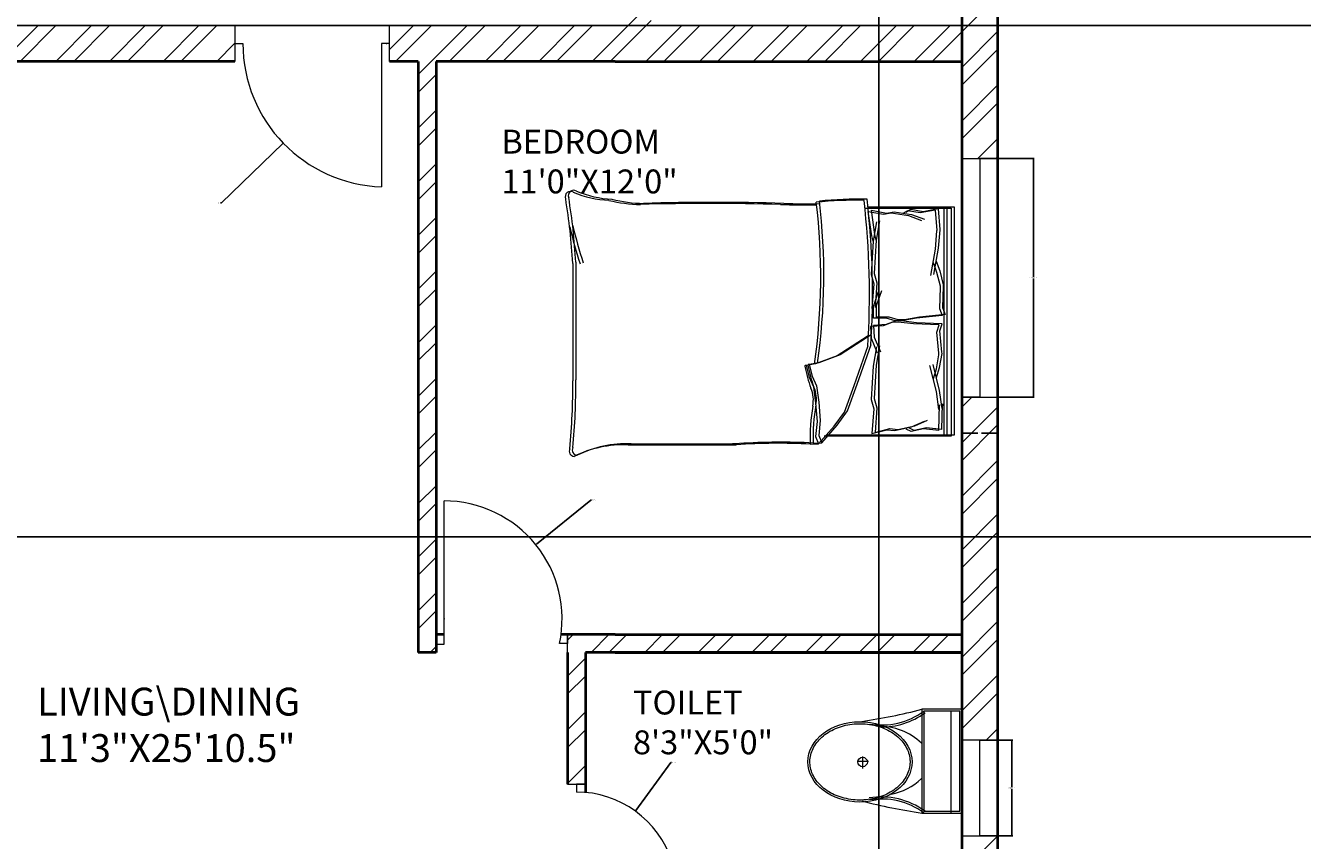
# Model space of a CAD drawing. Units: inches. Extents: x 1355 to 2746, y 1171 to 2751.
# Tile 4 of 24: x 1697 to 2017, y 1482 to 1686. Entities that reach past the tile are written whole.
import ezdxf

# ---------------------------------------------------------------- set-up
doc = ezdxf.new("R2010")
doc.units = ezdxf.units.IN
for name, color, linetype, lineweight in [('A-ANNO-DIMS', 2, 'Continuous', 18), ('A-AREA-IDEN', 7, 'Continuous', 18), ('A-DOOR', 3, 'Continuous', 20), ('A-FLOR-FIXT', 9, 'Continuous', 18), ('A-FURN', 8, 'Continuous', 13), ('A-GLAZ', 4, 'Continuous', 18), ('A-WALL', 7, 'Continuous', 40), ('A-WALL-PATT', 252, 'Continuous', 13)]:
    doc.layers.add(name, color=color, linetype=linetype, lineweight=lineweight)
doc.styles.get("Standard").update_dxf_attribs({"font": 'arial.ttf'})
doc.dimstyles.get("Standard").update_dxf_attribs({"dimtxt": 0.18, "dimasz": 0.18, "dimexe": 0.18, "dimexo": 0.0625, "dimgap": 0.09, "dimtad": 0, "dimtih": 1, "dimtoh": 1, "dimdec": 4, "dimzin": 0, "dimdsep": 46, "dimtxsty": 'Standard', "dimcen": 0.09, "dimadec": 0, "dimazin": 0, "dimtfac": 1, "dimtdec": 4, "dimtofl": 0, "dimtmove": 0, "dimatfit": 3, "dimfxl": 1, "dimtolj": 1, "dimtzin": 0, "dimarcsym": 0})

# ---------------------------------------------------------------- blocks, each defined once
blk = doc.blocks.new('A$C31115884')
for p, q in [((257.5, 466.4), (257.5, 523.2)), ((283.1, 497.7), (223.4, 497.7)), ((0, 200), (0, 0)), ((520, 200), (0, 200)), ((520, 0), (520, 200)), ((10, 190), (10, 10)), ((510, 190), (10, 190)), ((510, 10), (510, 190)), ((510, 54.5), (0, 54.5)), ((10, 10), (510, 10)), ((0, 0), (520, 0))]:
    blk.add_line(p, q)
blk.add_circle((255.6, 496.4), 23.6)
for centre, radius, start, end in [((2777.7, -204.6), 2807, 165.4549, 171.71327), ((-294.5, 403.3), 364.7, 324.20913, 9.34987), ((-294.5, 403.3), 374.7, 324.20913, 9.34987), ((805.8, 403.3), 364.7, 170.65013, 215.79087), ((3237, 905), 2807, 188.28673, 194.5451), ((139.5, 406.2), 293.5, 315.84364, 2.65635), ((805.8, 403.3), 374.7, 179.20365, 215.79087), ((383.6, 406.2), 293.5, 190.27735, 224.15636)]:
    blk.add_arc(centre, radius, start, end)
blk.add_ellipse((256.2, 509.9), major_axis=(0, -260.7), ratio=0.772727)
blk.add_open_spline([(256.2, 259.2), (263.1, 259.2), (270, 259.7), (287.8, 262.3), (298.7, 265.1), (319.9, 273.1), (330.2, 278.4), (350.1, 291.1), (359.7, 298.7), (377.7, 315.9), (386.2, 325.5), (401.7, 346.6), (408.8, 358.1), (421.3, 382.5), (426.8, 395.5), (435.9, 422.4), (439.5, 436.4), (444.8, 465.1), (446.5, 479.7), (447.9, 509.2), (447.6, 524), (445, 553.3), (442.7, 567.8), (436.3, 596), (432.1, 609.7), (421.9, 636), (416, 648.6), (402.5, 672.1), (395, 683), (378.6, 703), (369.8, 712.1), (351.1, 728), (341.3, 734.8), (320.9, 746.2), (310.4, 750.7), (288.9, 757.3), (278, 759.4), (256, 761), (245, 760.6), (223.1, 757.2), (212.3, 754.3), (191.1, 746.1), (180.8, 740.7), (160.9, 727.8), (151.4, 720.1), (133.5, 702.7), (125.1, 693), (109.6, 671.7), (102.6, 660.2), (90.2, 635.7), (84.9, 622.7), (76, 595.6), (72.4, 581.6), (67.2, 552.9), (65.6, 538.2), (64.4, 508.8), (64.8, 494), (67.5, 464.7), (69.9, 450.2), (76.6, 422), (80.8, 408.3), (91.1, 382.2), (97.2, 369.7), (110.8, 346.3), (118.4, 335.4), (134.8, 315.6), (143.7, 306.7), (162.4, 290.9), (172.3, 284.2), (192.8, 273), (203.3, 268.6), (224.8, 262.2), (235.8, 260.2), (249.9, 259.3), (253, 259.2), (256.2, 259.2)], degree=3, knots=[0, 0, 0, 0, 0.110105, 0.110105, 0.285049, 0.285049, 0.459994, 0.459994, 0.634938, 0.634938, 0.809882, 0.809882, 0.984827, 0.984827, 1.159771, 1.159771, 1.334715, 1.334715, 1.50966, 1.50966, 1.684604, 1.684604, 1.859549, 1.859549, 2.034493, 2.034493, 2.209437, 2.209437, 2.384382, 2.384382, 2.559326, 2.559326, 2.73427, 2.73427, 2.909215, 2.909215, 3.084159, 3.084159, 3.259103, 3.259103, 3.434048, 3.434048, 3.608992, 3.608992, 3.783936, 3.783936, 3.958881, 3.958881, 4.133825, 4.133825, 4.30877, 4.30877, 4.483714, 4.483714, 4.658658, 4.658658, 4.833603, 4.833603, 5.008547, 5.008547, 5.183491, 5.183491, 5.358436, 5.358436, 5.53338, 5.53338, 5.708324, 5.708324, 5.883269, 5.883269, 6.058213, 6.058213, 6.233158, 6.233158, 6.283185, 6.283185, 6.283185, 6.283185])
blk = doc.blocks.new('BED-DOUBLE-PLAN')
for p, q in [((75.16, 62.38), (96.87, 62.38)), ((75.93, 62.66), (97.64, 62.66)), ((76.95, 55.42), (76.08, 61.53)), ((76.08, 61.53), (79.9, 60.84)), ((77.72, 55.7), (76.85, 61.81)), ((76.85, 61.81), (80.66, 61.11)), ((79.9, 60.84), (81.8, 61.19)), ((80.66, 61.11), (82.57, 61.46)), ((81.8, 61.19), (86.14, 60.49)), ((82.57, 61.46), (86.9, 60.77)), ((85.96, 61.71), (84.75, 61.01)), ((86.73, 61.98), (85.52, 61.29)), ((89.08, 61.19), (85.96, 61.71)), ((89.85, 61.46), (86.73, 61.98)), ((92.9, 61.88), (89.08, 61.19)), ((93.66, 62.15), (89.85, 61.46)), ((92.87, 61.87), (93.27, 56.74)), ((93.64, 62.15), (94.03, 57.02)), ((95.03, 62.38), (95.03, 5.09)), ((95.8, 62.66), (95.8, 5.36)), ((96.87, 62.38), (96.87, 5.09)), ((97.64, 62.66), (97.64, 5.36)), ((78.14, 58.9), (77.34, 54.06)), ((78.9, 59.17), (78.1, 54.34)), ((86.14, 60.49), (89.43, 59.28)), ((86.9, 60.77), (90.2, 59.55)), ((77.34, 54.06), (76.95, 55.42)), ((78.1, 54.34), (77.72, 55.7)), ((93.24, 56.62), (92.9, 52.03)), ((93.27, 56.74), (93.24, 56.62)), ((94.01, 56.89), (93.66, 52.31)), ((94.03, 57.02), (94.01, 56.89)), ((77.34, 54.06), (76.82, 45.66)), ((78.1, 54.34), (77.59, 45.93)), ((92.9, 52.03), (91.68, 45.45)), ((93.66, 52.31), (92.45, 45.72)), ((1.87, 48.49), (1.87, 18.98)), ((2.64, 48.76), (2.64, 19.26)), ((92.38, 48.74), (93.24, 46.31)), ((93.14, 49.01), (94.01, 46.59)), ((76.82, 45.66), (77.49, 43.31)), ((77.59, 45.93), (78.25, 43.58)), ((93.24, 46.31), (94.11, 42.85)), ((94.01, 46.59), (94.88, 43.12)), ((77.49, 43.31), (77, 37.16)), ((78.25, 43.58), (77.77, 37.43)), ((78.14, 37.93), (79.45, 41.7)), ((94.11, 42.46), (93.94, 37.13)), ((94.11, 42.85), (94.11, 42.46)), ((94.88, 42.74), (94.7, 37.41)), ((94.88, 43.12), (94.88, 42.74)), ((77.38, 37.65), (78.68, 41.42)), ((77.38, 34.71), (77.38, 37.65)), ((78.14, 34.98), (78.14, 37.93)), ((94.63, 35.4), (88.22, 34.71)), ((95.4, 35.67), (88.98, 34.98)), ((93.94, 37.13), (94.63, 35.4)), ((94.7, 37.41), (95.4, 35.67)), ((79.83, 32.82), (76.62, 32.62)), ((76.62, 32.62), (76.8, 29.68)), ((80.59, 34.71), (77.38, 34.71)), ((80.6, 33.1), (77.39, 32.9)), ((77.39, 32.9), (77.57, 29.96)), ((81.36, 34.98), (78.14, 34.98)), ((82.03, 33.66), (79.83, 32.82)), ((82.84, 34.01), (80.59, 34.71)), ((82.8, 33.93), (80.6, 33.1)), ((83.61, 34.29), (81.36, 34.98)), ((83.59, 33.75), (82.03, 33.66)), ((84.36, 34.03), (82.8, 33.93)), ((84.4, 34.01), (82.84, 34.01)), ((87.44, 33.3), (83.59, 33.75)), ((85.17, 34.29), (83.61, 34.29)), ((88.21, 33.57), (84.36, 34.03)), ((88.22, 34.71), (84.4, 34.01)), ((88.98, 34.98), (85.17, 34.29)), ((93.89, 33.01), (87.44, 33.3)), ((94.65, 33.28), (88.21, 33.57)), ((93.3, 31.24), (93.89, 33.01)), ((94.07, 31.51), (94.65, 33.28)), ((76.03, 30.27), (68.25, 25.25)), ((76.8, 30.55), (69.01, 25.52)), ((76.8, 29.68), (78.34, 26)), ((77.57, 29.96), (79.11, 26.28)), ((93.81, 25.93), (93.3, 31.24)), ((94.57, 26.2), (94.07, 31.51)), ((72.52, 17.82), (76.03, 27.82)), ((73.28, 18.1), (76.8, 28.09)), ((78.14, 27.51), (77.34, 22.68)), ((78.9, 27.78), (78.1, 22.95)), ((93.83, 25.54), (93.81, 25.93)), ((93.95, 22.3), (94.6, 25.82)), ((94.6, 25.82), (94.57, 26.2)), ((62.87, 23.21), (60.45, 22.84)), ((60.45, 22.84), (61.2, 19.86)), ((63.63, 23.48), (61.22, 23.11)), ((61.22, 23.11), (61.96, 20.14)), ((68.25, 25.25), (62.87, 23.21)), ((69.01, 25.52), (63.63, 23.48)), ((77.34, 22.68), (76.82, 14.27)), ((78.1, 22.95), (77.59, 14.54)), ((93.19, 16.3), (91.57, 22.8)), ((93.96, 16.57), (92.34, 23.07)), ((93.18, 22.03), (93.83, 25.54)), ((61.2, 19.86), (62.31, 17.45)), ((61.96, 20.14), (63.08, 17.72)), ((92.47, 19.55), (93.18, 22.03)), ((93.23, 19.83), (93.95, 22.3)), ((62.31, 17.45), (62.87, 13.37)), ((63.08, 17.72), (63.63, 13.64)), ((70.1, 11.14), (72.52, 17.82)), ((70.87, 11.41), (73.28, 18.1)), ((93.82, 11.75), (93.19, 16.3)), ((94.59, 12.02), (93.96, 16.57)), ((62.87, 13.37), (63.24, 8.72)), ((63.63, 13.64), (64, 9)), ((76.82, 14.27), (77.49, 11.92)), ((77.59, 14.54), (78.25, 12.19)), ((93.81, 6.47), (93.92, 12.95)), ((93.92, 12.95), (93.82, 11.75)), ((94.57, 6.75), (94.69, 13.22)), ((94.69, 13.22), (94.59, 12.02)), ((67.51, 7.61), (70.1, 11.14)), ((68.27, 7.88), (70.87, 11.41)), ((77.49, 11.92), (77, 5.77)), ((78.25, 12.19), (77.77, 6.04)), ((63.24, 8.72), (62.87, 5.01)), ((63.61, 3.17), (67.51, 7.61)), ((64, 9), (63.63, 5.28)), ((64.38, 3.44), (68.27, 7.88)), ((77, 5.77), (80.77, 6.7)), ((77.77, 6.04), (81.53, 6.97)), ((80.77, 6.7), (82.69, 6.47)), ((81.53, 6.97), (83.46, 6.75)), ((82.69, 6.47), (86.97, 7.43)), ((83.46, 6.75), (87.74, 7.71)), ((86.88, 6.21), (85.62, 6.83)), ((87.64, 6.49), (86.39, 7.1)), ((89.96, 6.93), (86.88, 6.21)), ((86.97, 7.43), (90.18, 8.85)), ((90.72, 7.2), (87.64, 6.49)), ((87.74, 7.71), (90.95, 9.12)), ((93.81, 6.47), (89.96, 6.93)), ((94.57, 6.75), (90.72, 7.2)), ((62.28, 3.35), (64.38, 3.44, 4.64)), ((62.87, 5.01), (63.61, 3.17)), ((63.63, 5.28), (64.38, 3.44)), ((96.87, 5.09), (64.97, 5.09)), ((97.64, 5.36), (65.74, 5.36)), ((61.52, 3.07), (63.61, 3.17, 4.64))]:
    blk.add_line(p, q)
for centre, radius, start, end in [((1.3, 65.24), 1.31, 56.1736, 203.4781), ((-143.9, 40.86), 145.97, 2.9958, 9.4091), ((2.07, 65.52), 1.31, 56.1736, 203.4781), ((-143.14, 41.13), 145.97, 2.9958, 9.4091), ((12.62, 92.52), 28.25, 247.9751, 266.652), ((13.39, 92.79), 28.25, 247.9751, 266.652), ((19.53, 98.8), 35.53, 256.0648, 268.9113), ((20.29, 99.07), 35.53, 256.0648, 268.9113), ((72.78, -35.55), 99.87, 88.7218, 95.604), ((73.55, -35.27), 99.87, 88.7218, 95.604), ((-121.38, 40.94), 197.77, 356.0865, 6.7821), ((-120.62, 41.22), 197.77, 356.0865, 6.7821), ((36.19, -514.68), 578.22, 88.22771, 91.71854), ((36.96, -514.41), 578.22, 88.22771, 91.71854), ((59.5, 267.13), 203.94, 268.4762, 271.0082), ((60.27, 267.4), 203.94, 268.4762, 271.0082), ((-90.53, 45.26), 154.68, 351.7845, 6.9006), ((-89.76, 45.54), 154.68, 351.7845, 6.9006), ((126.07, 87.47), 127.63, 193.3832, 197.7053), ((125.3, 87.2), 127.63, 193.3832, 197.7053), ((60.38, 22.63), 0.221, 70.2464, 181.1377), ((95.1, 29.2), 35.55, 190.6617, 199.8806), ((61.15, 22.9), 0.221, 70.2464, 181.1377), ((95.86, 29.47), 35.55, 190.6617, 199.8806), ((-156.85, 17.49), 159.5, 354.4998, 0.6351), ((-157.62, 17.21), 159.5, 354.4998, 0.6351), ((54.83, 14.11), 7.46, 348.6608, 23.7384), ((55.6, 14.38), 7.46, 348.6608, 23.7384), ((105.62, 5.29), 43.38, 169.8763, 182.5657), ((104.85, 5.01), 43.38, 169.8763, 182.5657), ((16.33, 5472.16), 5469.02, 270.00217, 270.28689), ((53.34, -151.96), 155.25, 86.9791, 93.8365), ((54.1, -151.69), 155.25, 86.9791, 93.8365), ((2.32, 1.32), 1.32, 152.6588, 266.02), ((3.08, 1.59), 1.32, 152.6588, 266.02), ((14.55, -24.75), 27.65, 87.4714, 116.4681), ((15.32, -24.48), 27.65, 87.4714, 116.4681), ((15.56, 5471.89), 5469.02, 270.00217, 270.28689)]:
    blk.add_arc(centre, radius, start, end)
blk = doc.blocks.new('WINDOW-PLAN-60')
for p, q in [((0, 60), (9, 60)), ((9, 60), (4.5, 60)), ((4.5, 60), (4.5, 0)), ((4.5, 0), (0, 0)), ((0, 0), (9, 0))]:
    blk.add_line(p, q)
blk = doc.blocks.new('WINDOW-PLAN-24-3')
for p, q in [((9, 24), (0, 24)), ((0, 24), (0, 24)), ((4.5, 0), (4.5, 24)), ((4.5, 24), (9, 24)), ((0, 0), (9, 0)), ((9, 0), (4.5, 0))]:
    blk.add_line(p, q)
blk = doc.blocks.new('DOOR-BED-SE')
for p, q in [((2, 2.1), (2, 38.1)), ((33, 0), (33, 4.5)), ((33, 4.5), (33, 2.25)), ((0, 2.1), (2, 2.1)), ((33, 2.25), (31, 2.25))]:
    blk.add_line(p, q)
blk.add_arc((2, 8.44), 29.65, 347.948, 90)
blk = doc.blocks.new('DOOR-WC-SE')
for p, q in [((0, 21.41), (4.5, 21.41)), ((4.5, 21.41), (2.25, 21.41)), ((2.25, 21.41), (2.25, 19.41)), ((2.25, 0), (2.25, 2)), ((2.25, 2), (26.25, 2)), ((4.5, 0), (0, 0)), ((0, 0), (2.25, 0))]:
    blk.add_line(p, q)
blk.add_arc((2.25, -5.83), 25.25, 18.0786, 90)
blk = doc.blocks.new('DOOR-ENTRY-S')
for p, q in [((0, 40.5), (0, 31.5)), ((38.81, 31.5), (38.81, 40.5)), ((0, 36), (2, 36)), ((38.81, 36), (36.81, 36)), ((36.81, 36), (36.81, 0))]:
    blk.add_line(p, q)
blk.add_arc((38.02, 36), 36.02, 180, 268.0706)
blk = doc.blocks.new('*D39')
at = {"layer": 'A-ANNO-DIMS', "color": 0, "lineweight": -2, "transparency": 16777216}
for p, q in [((1940.77, 1652.94), (1949.89, 1652.94)), ((1949.71, 1652.76), (1949.71, 1623.13)), ((1949.71, 1593.12), (1949.71, 1622.76)), ((1940.77, 1592.94), (1949.89, 1592.94))]:
    blk.add_line(p, q, dxfattribs=at)
at = {"layer": 'A-ANNO-DIMS', "color": 0, "transparency": 16777216}
for points in [[(1949.68, 1652.76), (1949.74, 1652.76), (1949.71, 1652.94)], [(1949.68, 1593.12), (1949.74, 1593.12), (1949.71, 1592.94)]]:
    blk.add_solid(points, dxfattribs=at)
at = {"layer": 'Defpoints', "color": 0, "transparency": 16777216}
for p in [(1940.71, 1652.94), (1949.71, 1652.94), (1940.71, 1592.94)]:
    blk.add_point(p, dxfattribs=at)
at = {"layer": 'A-ANNO-DIMS', "color": 0, "transparency": 16777216, "insert": (1949.71, 1622.94), "char_height": 0.18, "attachment_point": 5}
blk.add_mtext('\\A1;WINDOW 60 TYP.', dxfattribs=at)
blk = doc.blocks.new('*D40')
at = {"layer": 'A-ANNO-DIMS', "color": 0, "lineweight": -2, "transparency": 16777216}
for p, q in [((1931.71, 1592.88), (1931.71, 1583.76)), ((1940.71, 1592.88), (1940.71, 1583.76)), ((1931.89, 1583.94), (1935.75, 1583.94)), ((1940.53, 1583.94), (1936.67, 1583.94))]:
    blk.add_line(p, q, dxfattribs=at)
at = {"layer": 'A-ANNO-DIMS', "color": 0, "transparency": 16777216}
for points in [[(1931.89, 1583.97), (1931.89, 1583.91), (1931.71, 1583.94)], [(1940.53, 1583.97), (1940.53, 1583.91), (1940.71, 1583.94)]]:
    blk.add_solid(points, dxfattribs=at)
at = {"layer": 'Defpoints', "color": 0, "transparency": 16777216}
for p in [(1931.71, 1592.94), (1940.71, 1592.94), (1940.71, 1583.94)]:
    blk.add_point(p, dxfattribs=at)
at = {"layer": 'A-ANNO-DIMS', "color": 0, "transparency": 16777216, "insert": (1936.21, 1583.94), "char_height": 0.18, "attachment_point": 5}
blk.add_mtext('\\A1;9 TYP.', dxfattribs=at)
blk = doc.blocks.new('*D51')
at = {"layer": 'A-ANNO-DIMS', "color": 0, "lineweight": -2, "transparency": 16777216}
for p, q in [((1940.77, 1506.78), (1944.49, 1506.78)), ((1944.31, 1506.6), (1944.31, 1494.97)), ((1944.31, 1482.96), (1944.31, 1494.6)), ((1940.77, 1482.78), (1944.49, 1482.78))]:
    blk.add_line(p, q, dxfattribs=at)
at = {"layer": 'A-ANNO-DIMS', "color": 0, "transparency": 16777216}
for points in [[(1944.28, 1506.6), (1944.34, 1506.6), (1944.31, 1506.78)], [(1944.28, 1482.96), (1944.34, 1482.96), (1944.31, 1482.78)]]:
    blk.add_solid(points, dxfattribs=at)
at = {"layer": 'Defpoints', "color": 0, "transparency": 16777216}
for p in [(1940.71, 1506.78), (1944.31, 1506.78), (1940.71, 1482.78)]:
    blk.add_point(p, dxfattribs=at)
at = {"layer": 'A-ANNO-DIMS', "color": 0, "transparency": 16777216, "insert": (1944.31, 1494.78), "char_height": 0.18, "attachment_point": 5}
blk.add_mtext('\\A1;WINDOW 24 TYP.', dxfattribs=at)
blk = doc.blocks.new('*D52')
at = {"layer": 'A-ANNO-DIMS', "color": 0, "lineweight": -2, "transparency": 16777216}
for p, q in [((1931.71, 1482.72), (1931.71, 1479)), ((1940.71, 1482.72), (1940.71, 1479)), ((1931.89, 1479.18), (1935.75, 1479.18)), ((1940.53, 1479.18), (1936.67, 1479.18))]:
    blk.add_line(p, q, dxfattribs=at)
at = {"layer": 'A-ANNO-DIMS', "color": 0, "transparency": 16777216}
for points in [[(1931.89, 1479.21), (1931.89, 1479.15), (1931.71, 1479.18)], [(1940.53, 1479.21), (1940.53, 1479.15), (1940.71, 1479.18)]]:
    blk.add_solid(points, dxfattribs=at)
at = {"layer": 'Defpoints', "color": 0, "transparency": 16777216}
for p in [(1931.71, 1482.78), (1940.71, 1482.78), (1940.71, 1479.18)]:
    blk.add_point(p, dxfattribs=at)
at = {"layer": 'A-ANNO-DIMS', "color": 0, "transparency": 16777216, "insert": (1936.21, 1479.18), "char_height": 0.18, "attachment_point": 5}
blk.add_mtext('\\A1;9 TYP.', dxfattribs=at)
blk = doc.blocks.new('*D106')
at = {"layer": 'A-ANNO-DIMS', "color": 0, "lineweight": -2, "transparency": 16777216}
for p, q in [((2031.09, 1557.85), (1407.53, 1557.85)), ((1407.71, 1557.67), (1407.71, 1434.76)), ((1407.71, 1311.48), (1407.71, 1434.39)), ((2080.33, 1311.3), (1407.53, 1311.3))]:
    blk.add_line(p, q, dxfattribs=at)
at = {"layer": 'A-ANNO-DIMS', "color": 0, "transparency": 16777216}
for points in [[(1407.68, 1557.67), (1407.74, 1557.67), (1407.71, 1557.85)], [(1407.68, 1311.48), (1407.74, 1311.48), (1407.71, 1311.3)]]:
    blk.add_solid(points, dxfattribs=at)
at = {"layer": 'Defpoints', "color": 0, "transparency": 16777216}
for p in [(1407.71, 1557.85), (2031.15, 1557.85), (2080.39, 1311.3)]:
    blk.add_point(p, dxfattribs=at)
at = {"layer": 'A-ANNO-DIMS', "color": 0, "transparency": 16777216, "insert": (1407.71, 1434.57), "char_height": 0.18, "attachment_point": 5}
blk.add_mtext('\\A1;246.54', dxfattribs=at)
blk = doc.blocks.new('*D107')
at = {"layer": 'A-ANNO-DIMS', "color": 0, "lineweight": -2, "transparency": 16777216}
for p, q in [((2089.33, 1686.3), (1407.53, 1686.3)), ((1407.71, 1686.12), (1407.71, 1622.26)), ((1407.71, 1558.03), (1407.71, 1621.89)), ((2031.09, 1557.85), (1407.53, 1557.85))]:
    blk.add_line(p, q, dxfattribs=at)
at = {"layer": 'A-ANNO-DIMS', "color": 0, "transparency": 16777216}
for points in [[(1407.68, 1686.12), (1407.74, 1686.12), (1407.71, 1686.3)], [(1407.68, 1558.03), (1407.74, 1558.03), (1407.71, 1557.85)]]:
    blk.add_solid(points, dxfattribs=at)
at = {"layer": 'Defpoints', "color": 0, "transparency": 16777216}
for p in [(1407.71, 1686.3), (2089.39, 1686.3), (2031.15, 1557.85)]:
    blk.add_point(p, dxfattribs=at)
at = {"layer": 'A-ANNO-DIMS', "color": 0, "transparency": 16777216, "insert": (1407.71, 1622.07), "char_height": 0.18, "attachment_point": 5}
blk.add_mtext('\\A1;128.46', dxfattribs=at)
blk = doc.blocks.new('*D145')
at = {"layer": 'A-ANNO-DIMS', "color": 0, "lineweight": -2, "transparency": 16777216}
for p, q in [((1910.88, 1399.86), (1910.88, 2716.58)), ((1911.06, 2716.4), (1920.83, 2716.4)), ((1931.53, 2716.4), (1921.76, 2716.4)), ((1931.71, 1399.86), (1931.71, 2716.58))]:
    blk.add_line(p, q, dxfattribs=at)
at = {"layer": 'A-ANNO-DIMS', "color": 0, "transparency": 16777216}
for points in [[(1911.06, 2716.43), (1911.06, 2716.37), (1910.88, 2716.4)], [(1931.53, 2716.43), (1931.53, 2716.37), (1931.71, 2716.4)]]:
    blk.add_solid(points, dxfattribs=at)
at = {"layer": 'Defpoints', "color": 0, "transparency": 16777216}
for p in [(1931.71, 2716.4), (1910.88, 1399.8), (1931.71, 1399.8)]:
    blk.add_point(p, dxfattribs=at)
at = {"layer": 'A-ANNO-DIMS', "color": 0, "transparency": 16777216, "insert": (1921.3, 2716.4), "char_height": 0.18, "attachment_point": 5}
blk.add_mtext('\\A1;20.824', dxfattribs=at)
blk = doc.blocks.new('*D155')
at = {"layer": 'A-ANNO-DIMS', "color": 0, "lineweight": -2, "transparency": 16777216}
for p, q in [((1787.15, 1681.8), (1787.33, 1681.8)), ((1787.24, 1681.71), (1787.24, 1681.89)), ((1745.81, 1641.74), (1761.22, 1656.64)), ((1745.63, 1641.74), (1745.81, 1641.74))]:
    blk.add_line(p, q, dxfattribs=at)
at = {"layer": 'A-ANNO-DIMS', "color": 0, "transparency": 16777216}
blk.add_solid([(1761.19, 1656.66), (1761.24, 1656.62), (1761.34, 1656.76)], dxfattribs=at)
at = {"layer": 'Defpoints', "color": 0, "transparency": 16777216}
for p in [(1787.24, 1681.8), (1761.34, 1656.76)]:
    blk.add_point(p, dxfattribs=at)
at = {"layer": 'A-ANNO-DIMS', "color": 0, "transparency": 16777216, "insert": (1745.15, 1641.74), "char_height": 0.18, "attachment_point": 5}
blk.add_mtext('\\A1;R36.02', dxfattribs=at)
blk = doc.blocks.new('*D157')
at = {"layer": 'A-ANNO-DIMS', "color": 0, "lineweight": -2, "transparency": 16777216}
for p, q in [((1838.59, 1567.09), (1824.9, 1556.01)), ((1838.77, 1567.09), (1838.59, 1567.09)), ((1801.62, 1537.24), (1801.8, 1537.24)), ((1801.71, 1537.15), (1801.71, 1537.33))]:
    blk.add_line(p, q, dxfattribs=at)
at = {"layer": 'A-ANNO-DIMS', "color": 0, "transparency": 16777216}
blk.add_solid([(1824.88, 1556.03), (1824.92, 1555.98), (1824.76, 1555.89)], dxfattribs=at)
at = {"layer": 'Defpoints', "color": 0, "transparency": 16777216}
for p in [(1824.76, 1555.89), (1801.71, 1537.24)]:
    blk.add_point(p, dxfattribs=at)
at = {"layer": 'A-ANNO-DIMS', "color": 0, "transparency": 16777216, "insert": (1839.32, 1567.09), "char_height": 0.18, "attachment_point": 5}
blk.add_mtext('\\A1;R29.654', dxfattribs=at)
blk = doc.blocks.new('*D161')
at = {"layer": 'A-ANNO-DIMS', "color": 0, "lineweight": -2, "transparency": 16777216}
for p, q in [((1858.68, 1501.2), (1849.89, 1489.09)), ((1858.86, 1501.2), (1858.68, 1501.2)), ((1834.87, 1468.51), (1835.05, 1468.51)), ((1834.96, 1468.42), (1834.96, 1468.6))]:
    blk.add_line(p, q, dxfattribs=at)
at = {"layer": 'A-ANNO-DIMS', "color": 0, "transparency": 16777216}
blk.add_solid([(1849.87, 1489.1), (1849.91, 1489.07), (1849.78, 1488.94)], dxfattribs=at)
at = {"layer": 'Defpoints', "color": 0, "transparency": 16777216}
for p in [(1849.78, 1488.94), (1834.96, 1468.51)]:
    blk.add_point(p, dxfattribs=at)
at = {"layer": 'A-ANNO-DIMS', "color": 0, "transparency": 16777216, "insert": (1859.41, 1501.2), "char_height": 0.18, "attachment_point": 5}
blk.add_mtext('\\A1;R25.246', dxfattribs=at)

msp = doc.modelspace()

# ---------------------------------------------------------------- hatches: boundary and pattern name
at = {"layer": 'A-WALL-PATT'}
h = msp.add_hatch(dxfattribs=at)
h.set_pattern_fill('ANSI32', color=256)
h.paths.add_polyline_path([(1660.2083, 2139.3018), (1614.5977, 2139.3018), (1614.5977, 2130.3018), (1655.7083, 2130.3018), (1655.7083, 1981.8018), (1660.2083, 1981.8018), (1660.2083, 2090.7225), (1692.5832, 2090.7225), (1692.5832, 2095.2225), (1660.2083, 2095.2225)])
h.paths.add_polyline_path([(1523.7083, 2130.3018), (1554.5977, 2130.3018), (1554.5977, 2134.8018), (1554.5977, 2139.3018), (1514.7083, 2139.3018), (1514.7083, 2071.8385), (1523.7083, 2071.8385)])
h.paths.add_polyline_path([(1940.7083, 2139.3018), (1883.7928, 2139.3018), (1883.7928, 2130.3018), (1931.7083, 2130.3018), (1931.7083, 2098.3333), (1940.7083, 2098.3333)])
h.paths.add_polyline_path([(1799.7083, 2130.3018), (1823.7928, 2130.3018), (1823.7928, 2134.8018), (1823.7928, 2139.3018), (1795.2083, 2139.3018), (1795.2083, 2130.3018), (1795.2083, 2095.2225), (1759.2134, 2095.2225), (1759.2134, 2090.7225), (1795.2083, 2090.7225), (1795.2083, 1981.8018), (1799.7083, 1981.8018), (1799.7083, 1986.3018)])
h.paths.add_polyline_path([(1940.7083, 2038.3333), (1931.7083, 2038.3333), (1931.7083, 1986.3018), (1832.7083, 1986.3018), (1832.7083, 1947.1338), (1837.2083, 1947.1338), (1837.2083, 1981.8018), (1931.7083, 1981.8018), (1931.7083, 1967.1939), (1940.7083, 1967.1939)])
h.paths.add_polyline_path([(1940.7083, 1943.1939), (1931.7083, 1943.1939), (1931.7083, 1921.8018), (1837.2083, 1921.8018), (1837.2083, 1926.0511), (1832.7083, 1926.0511), (1832.7083, 1917.3018), (1931.7083, 1917.3018), (1931.7083, 1908.3321), (1940.7083, 1908.3321)])
h.paths.add_polyline_path([(1940.7083, 1884.3321), (1931.7083, 1884.3321), (1931.7083, 1869.3018), (1899.4583, 1869.3018), (1899.4583, 1864.8018), (1931.7083, 1864.8018), (1931.7083, 1773.3018), (1786.5143, 1773.3018), (1786.5143, 1764.3018), (1844.7083, 1764.3018), (1844.7083, 1748.9343), (1853.7083, 1748.9343), (1853.7083, 1764.3018), (1931.7083, 1764.3018), (1931.7083, 1652.9424), (1940.7083, 1652.9424)])
h.paths.add_polyline_path([(1799.7083, 1864.8018), (1806.0522, 1864.8018), (1806.0522, 1867.0518), (1806.0522, 1869.3018), (1799.7083, 1869.3018), (1799.7083, 1917.3018), (1799.7083, 1921.8018), (1795.2083, 1921.8018), (1795.2083, 1773.3018), (1799.7083, 1773.3018)])
h.paths.add_polyline_path([(1872.8988, 1867.0518), (1872.8988, 1869.3018), (1867.2083, 1869.3018), (1867.2083, 1917.3018), (1862.7083, 1917.3018), (1862.7083, 1869.3018), (1836.9546, 1869.3018), (1836.9546, 1864.8018), (1862.7083, 1864.8018), (1872.8988, 1864.8018)])
h.paths.add_polyline_path([(1749.2197, 1773.3018), (1655.7083, 1773.3018), (1523.7083, 1773.3018), (1523.7083, 1828.4963), (1514.7083, 1828.4963), (1514.7083, 1753.9033), (1519.2083, 1753.9033), (1523.7083, 1753.9033), (1523.7083, 1764.3018), (1655.7083, 1764.3018), (1749.2197, 1764.3018), (1749.2197, 1768.8018)])
h.paths.add_polyline_path([(1660.2083, 1921.8018), (1655.7083, 1921.8018), (1655.7083, 1917.3018), (1655.7083, 1773.3018), (1660.2083, 1773.3018)])
h.paths.add_polyline_path([(1523.7083, 2011.8385), (1514.7083, 2011.8385), (1514.7083, 1973.114), (1519.2083, 1973.114), (1523.7083, 1973.114), (1523.7083, 1976.8227), (1523.7083, 1981.8018), (1618.2083, 1981.8018), (1618.2083, 1921.8018), (1553.707, 1921.8018), (1553.707, 1917.3018), (1622.7083, 1917.3018), (1622.7083, 1919.5518), (1622.7083, 1921.8018), (1622.7083, 1986.3018), (1523.7083, 1986.3018)])
h.paths.add_polyline_path([(1529.6686, 1919.5518), (1529.6686, 1921.8018), (1523.7083, 1921.8018), (1523.7083, 1949.114), (1514.7083, 1949.114), (1514.7083, 1888.4963), (1523.7083, 1888.4963), (1523.7083, 1917.3018), (1529.6686, 1917.3018)])
h.paths.add_polyline_path([(1538.9419, 1775.643), (1585.5504, 1775.643), (1585.5504, 1798.0318), (1538.9419, 1798.0318)], flags=25)
h.paths.add_polyline_path([(1696.7097, 1497.3356), (1769.5651, 1497.3356), (1769.5651, 1523.4559), (1696.7097, 1523.4559)], flags=9)
h.paths.add_polyline_path([(1629.1643, 1230.5133), (1877.0879, 1230.5133), (1877.0879, 1267.606), (1629.1643, 1267.606)], flags=9)
h.paths.add_polyline_path([(2533.4462, 2215.4033), (2579.9292, 2215.4033), (2579.9292, 2231.889), (2533.4462, 2231.889)], flags=9)
h.paths.add_polyline_path([(2540.822, 2515.6945), (2594.2245, 2515.6945), (2594.2245, 2545.5463), (2540.822, 2545.5463)], flags=9)
h.paths.add_polyline_path([(2535.9857, 2588.2819), (2582.4687, 2588.2819), (2582.4687, 2604.7675), (2535.9857, 2604.7675)], flags=9)
h.paths.add_polyline_path([(2537.1627, 2617.1172), (2649.1245, 2617.1172), (2649.1245, 2633.6029), (2537.1627, 2633.6029)], flags=9)
h.paths.add_polyline_path([(2218.0051, 2168.228), (2363.9573, 2168.228), (2363.9573, 2205.3208), (2218.0051, 2205.3208)], flags=9)
h.paths.add_polyline_path([(1650.2156, 2165.3631), (1800.3547, 2165.3631), (1800.3547, 2202.4559), (1650.2156, 2202.4559)], flags=9)
h.paths.add_polyline_path([(2553.9592, 1610.7663), (2588.4203, 1610.7663), (2588.4203, 1660.2233), (2553.9592, 1660.2233)], flags=9)
h.paths.add_polyline_path([(1549.0868, 1648.2033), (1595.6952, 1648.2033), (1595.6952, 1670.5921), (1549.0868, 1670.5921)], flags=9)
h.paths.add_polyline_path([(1546.9525, 1502.0931), (1583.3413, 1502.0931), (1583.3413, 1524.4819), (1546.9525, 1524.4819)], flags=9)
h.paths.add_polyline_path([(1540.7704, 1433.4431), (1587.3788, 1433.4431), (1587.3788, 1455.8319), (1540.7704, 1455.8319)], flags=9)
h.paths.add_polyline_path([(1683.6524, 1321.5269), (1760.6169, 1321.5269), (1760.6169, 1333.8911), (1683.6524, 1333.8911)], flags=9)
h.paths.add_polyline_path([(1832.0485, 1356.0874), (1873.0989, 1356.0874), (1873.0989, 1378.4762), (1832.0485, 1378.4762)], flags=9)
h.paths.add_polyline_path([(1877.9694, 1431.2138), (1926.3827, 1431.2138), (1926.3827, 1453.578), (1877.9694, 1453.578)], flags=9)
h.paths.add_polyline_path([(1847.3106, 1499.8371), (1883.6994, 1499.8371), (1883.6994, 1522.2259), (1847.3106, 1522.2259)], flags=9)
h.paths.add_polyline_path([(1813.7015, 1640.7287), (1860.3099, 1640.7287), (1860.3099, 1663.1175), (1813.7015, 1663.1175)], flags=9)
h.paths.add_polyline_path([(1876.2576, 1710.2471), (1912.9452, 1710.2471), (1912.9452, 1732.6359), (1876.2576, 1732.6359)], flags=25)
h.paths.add_polyline_path([(1695.9163, 1715.3064), (1736.9668, 1715.3064), (1736.9668, 1737.6952), (1695.9163, 1737.6952)], flags=9)
h.paths.add_polyline_path([(1881.8583, 1888.9094), (1930.2717, 1888.9094), (1930.2717, 1911.2737), (1881.8583, 1911.2737)], flags=9)
h.paths.add_polyline_path([(1823.9298, 1798.6431), (1864.9803, 1798.6431), (1864.9803, 1821.0319), (1823.9298, 1821.0319)], flags=25)
h.paths.add_polyline_path([(1845.6062, 1948.1408), (1881.995, 1948.1408), (1881.995, 1970.5296), (1845.6062, 1970.5296)], flags=25)
h.paths.add_polyline_path([(1849.027, 1991.5151), (1895.6355, 1991.5151), (1895.6355, 2013.9039), (1849.027, 2013.9039)], flags=25)
h.paths.add_polyline_path([(1684.9725, 2113.8416), (1764.2658, 2113.8416), (1764.2658, 2126.2058), (1684.9725, 2126.2058)], flags=9)
h.paths.add_polyline_path([(1688.6193, 1913.0676), (1776.2005, 1913.0676), (1776.2005, 1935.4564), (1688.6193, 1935.4564)], flags=9)
h.paths.add_polyline_path([(1571.4689, 1930.9816), (1607.8577, 1930.9816), (1607.8577, 1953.3704), (1571.4689, 1953.3704)], flags=25)
h.paths.add_polyline_path([(1535.3581, 1998.3125), (1581.9665, 1998.3125), (1581.9665, 2020.7014), (1535.3581, 2020.7014)], flags=9)
h = msp.add_hatch(dxfattribs=at)
h.set_pattern_fill('ANSI32', color=256)
h.paths.add_polyline_path([(1749.2197, 1686.3018), (1732.6892, 1686.3018), (1523.7083, 1686.3018), (1523.7083, 1705.9033), (1514.7083, 1705.9033), (1514.7083, 1647.8732), (1519.2083, 1647.8732), (1523.7083, 1647.8732), (1523.7083, 1677.3018), (1655.7083, 1677.3018), (1655.7083, 1528.8018), (1660.2083, 1528.8018), (1660.2083, 1677.3018), (1732.6892, 1677.3018), (1749.2197, 1677.3018)])
h.paths.add_polyline_path([(1931.7083, 1686.3018), (1853.7083, 1686.3018), (1853.7083, 1703.5696), (1844.7083, 1703.5696), (1844.7083, 1686.3018), (1788.0274, 1686.3018), (1788.0274, 1677.3018), (1795.2083, 1677.3018), (1795.2083, 1528.8018), (1799.7083, 1528.8018), (1799.7083, 1677.3018), (1844.7083, 1677.3018), (1931.7083, 1677.3018)])
h.paths.add_polyline_path([(1931.7083, 1533.3018), (1844.7083, 1533.3018), (1832.7083, 1533.3018), (1832.7083, 1531.0518), (1832.7083, 1528.8018), (1832.7083, 1495.7519), (1837.2083, 1495.7519), (1837.2083, 1528.8018), (1931.7083, 1528.8018)])
h.paths.add_polyline_path([(1940.7083, 1592.9424), (1931.7083, 1592.9424), (1931.7083, 1506.7845), (1940.7083, 1506.7845)])
h.paths.add_polyline_path([(1940.7083, 1482.7845), (1936.2083, 1482.7845), (1931.7083, 1482.7845), (1931.7083, 1320.3018), (1880.7083, 1320.3018), (1880.7083, 1311.3018), (1940.7083, 1311.3018)])
h.paths.add_polyline_path([(1931.7083, 1468.8018), (1844.7083, 1468.8018), (1837.2083, 1468.8018), (1837.2083, 1474.34), (1832.7083, 1474.34), (1832.7083, 1468.8018), (1832.7083, 1464.3018), (1844.7083, 1464.3018), (1931.7083, 1464.3018)])
h.paths.add_polyline_path([(1863.8571, 1464.3018), (1859.3571, 1464.3018), (1859.3571, 1404.1662), (1838.1542, 1404.1662), (1838.1542, 1399.8018), (1869.4185, 1399.8018), (1869.4185, 1402.0518), (1869.4185, 1404.3018), (1863.8571, 1404.3018)])
h.paths.add_polyline_path([(1799.7083, 1399.6662), (1805.4082, 1399.6662), (1805.4082, 1401.9162), (1805.4082, 1404.1662), (1799.7083, 1404.1662), (1799.7083, 1464.3018), (1799.7083, 1468.8018), (1795.2083, 1468.8018), (1795.2083, 1356.2098), (1761.2597, 1356.2098), (1761.2597, 1351.7098), (1795.2083, 1351.7098), (1795.2083, 1320.3018), (1795.2083, 1311.3018), (1844.7083, 1311.3018), (1844.7083, 1315.8018), (1844.7083, 1320.3018), (1799.7083, 1320.3018)])
h.paths.add_polyline_path([(1692.9218, 1356.2098), (1660.2083, 1356.2098), (1660.2083, 1430.786), (1657.9583, 1430.786), (1655.7083, 1430.786), (1655.7083, 1320.3018), (1611.934, 1320.3018), (1611.934, 1311.3018), (1660.2083, 1311.3018), (1660.2083, 1351.7098), (1692.9218, 1351.7098)])
h.paths.add_polyline_path([(1523.7083, 1372.653), (1514.7083, 1372.653), (1514.7083, 1311.3018), (1551.934, 1311.3018), (1551.934, 1315.8018), (1551.934, 1320.3018), (1523.7083, 1320.3018)])
h.paths.add_polyline_path([(1523.7083, 1490.9023), (1514.7083, 1490.9023), (1514.7083, 1432.653), (1519.2083, 1432.653), (1523.7083, 1432.653)])
h.paths.add_polyline_path([(1660.2083, 1468.8018), (1622.7083, 1468.8018), (1622.7083, 1473.1566), (1618.2083, 1473.1566), (1618.2083, 1468.8018), (1523.7083, 1468.8018), (1523.7083, 1464.3018), (1655.7083, 1464.3018), (1655.7083, 1460.5634), (1660.2083, 1460.5634)])
h.paths.add_polyline_path([(1523.7083, 1587.8732), (1514.7083, 1587.8732), (1514.7083, 1514.9023), (1519.2083, 1514.9023), (1523.7083, 1514.9023)])
h.paths.add_polyline_path([(1622.7083, 1533.3018), (1523.7083, 1533.3018), (1523.7083, 1528.8018), (1618.2083, 1528.8018), (1618.2083, 1494.4205), (1622.7083, 1494.4205), (1622.7083, 1528.8018)])
h.paths.add_polyline_path([(1696.7097, 1497.3356), (1769.5651, 1497.3356), (1769.5651, 1523.4559), (1696.7097, 1523.4559)], flags=9)
h.paths.add_polyline_path([(1629.1643, 1230.5133), (1877.0879, 1230.5133), (1877.0879, 1267.606), (1629.1643, 1267.606)], flags=9)
h.paths.add_polyline_path([(2533.4462, 2215.4033), (2579.9292, 2215.4033), (2579.9292, 2231.889), (2533.4462, 2231.889)], flags=9)
h.paths.add_polyline_path([(2540.822, 2515.6945), (2594.2245, 2515.6945), (2594.2245, 2545.5463), (2540.822, 2545.5463)], flags=9)
h.paths.add_polyline_path([(2535.9857, 2588.2819), (2582.4687, 2588.2819), (2582.4687, 2604.7675), (2535.9857, 2604.7675)], flags=9)
h.paths.add_polyline_path([(2537.1627, 2617.1172), (2649.1245, 2617.1172), (2649.1245, 2633.6029), (2537.1627, 2633.6029)], flags=9)
h.paths.add_polyline_path([(2218.0051, 2168.228), (2363.9573, 2168.228), (2363.9573, 2205.3208), (2218.0051, 2205.3208)], flags=9)
h.paths.add_polyline_path([(1650.2156, 2165.3631), (1800.3547, 2165.3631), (1800.3547, 2202.4559), (1650.2156, 2202.4559)], flags=9)
h.paths.add_polyline_path([(2553.9592, 1610.7663), (2588.4203, 1610.7663), (2588.4203, 1660.2233), (2553.9592, 1660.2233)], flags=9)
h.paths.add_polyline_path([(1549.0868, 1648.2033), (1595.6952, 1648.2033), (1595.6952, 1670.5921), (1549.0868, 1670.5921)], flags=25)
h.paths.add_polyline_path([(1546.9525, 1502.0931), (1583.3413, 1502.0931), (1583.3413, 1524.4819), (1546.9525, 1524.4819)], flags=25)
h.paths.add_polyline_path([(1540.7704, 1433.4431), (1587.3788, 1433.4431), (1587.3788, 1455.8319), (1540.7704, 1455.8319)], flags=9)
h.paths.add_polyline_path([(1683.6524, 1321.5269), (1760.6169, 1321.5269), (1760.6169, 1333.8911), (1683.6524, 1333.8911)], flags=9)
h.paths.add_polyline_path([(1832.0485, 1356.0874), (1873.0989, 1356.0874), (1873.0989, 1378.4762), (1832.0485, 1378.4762)], flags=9)
h.paths.add_polyline_path([(1877.9694, 1431.2138), (1926.3827, 1431.2138), (1926.3827, 1453.578), (1877.9694, 1453.578)], flags=9)
h.paths.add_polyline_path([(1847.3106, 1499.8371), (1883.6994, 1499.8371), (1883.6994, 1522.2259), (1847.3106, 1522.2259)], flags=25)
h.paths.add_polyline_path([(1813.7015, 1640.7287), (1860.3099, 1640.7287), (1860.3099, 1663.1175), (1813.7015, 1663.1175)], flags=25)
h.paths.add_polyline_path([(1876.2576, 1710.2471), (1912.9452, 1710.2471), (1912.9452, 1732.6359), (1876.2576, 1732.6359)], flags=9)
h.paths.add_polyline_path([(1695.9163, 1715.3064), (1736.9668, 1715.3064), (1736.9668, 1737.6952), (1695.9163, 1737.6952)], flags=9)
h.paths.add_polyline_path([(1881.8583, 1888.9094), (1930.2717, 1888.9094), (1930.2717, 1911.2737), (1881.8583, 1911.2737)], flags=9)
h.paths.add_polyline_path([(1823.9298, 1798.6431), (1864.9803, 1798.6431), (1864.9803, 1821.0319), (1823.9298, 1821.0319)], flags=9)
h.paths.add_polyline_path([(1845.6062, 1948.1408), (1881.995, 1948.1408), (1881.995, 1970.5296), (1845.6062, 1970.5296)], flags=9)
h.paths.add_polyline_path([(1849.027, 1991.5151), (1895.6355, 1991.5151), (1895.6355, 2013.9039), (1849.027, 2013.9039)], flags=9)
h.paths.add_polyline_path([(1684.9725, 2113.8416), (1764.2658, 2113.8416), (1764.2658, 2126.2058), (1684.9725, 2126.2058)], flags=9)
h.paths.add_polyline_path([(1688.6193, 1913.0676), (1776.2005, 1913.0676), (1776.2005, 1935.4564), (1688.6193, 1935.4564)], flags=9)
h.paths.add_polyline_path([(1538.9419, 1775.643), (1585.5504, 1775.643), (1585.5504, 1798.0318), (1538.9419, 1798.0318)], flags=9)
h.paths.add_polyline_path([(1571.4689, 1930.9816), (1607.8577, 1930.9816), (1607.8577, 1953.3704), (1571.4689, 1953.3704)], flags=9)
h.paths.add_polyline_path([(1535.3581, 1998.3125), (1581.9665, 1998.3125), (1581.9665, 2020.7014), (1535.3581, 2020.7014)], flags=9)

# ---------------------------------------------------------------- linework, layer by layer
at = {"layer": 'A-WALL'}
for p, q in [((1940.7083, 2139.3018), (1940.7083, 1311.3018)), ((1931.7083, 1764.3018), (1931.7083, 1320.3018)), ((1732.6892, 1677.3018), (1660.2083, 1677.3018)), ((1749.2197, 1677.3018), (1732.6892, 1677.3018)), ((1795.2083, 1677.3018), (1788.0274, 1677.3018)), ((1795.2083, 1677.3018), (1795.2083, 1528.8018)), ((1799.7083, 1677.3018), (1799.7083, 1528.8018)), ((1844.7083, 1677.3018), (1799.7083, 1677.3018)), ((1844.7083, 1677.3018), (1931.7083, 1677.3018)), ((1801.7083, 1533.3018), (1799.7083, 1533.3018)), ((1844.7083, 1533.3018), (1831.0988, 1533.3018)), ((1844.7083, 1533.3018), (1931.7083, 1533.3018)), ((1799.7083, 1528.8018), (1795.2083, 1528.8018)), ((1832.7083, 1528.8018), (1832.7083, 1495.7519)), ((1844.7083, 1528.8018), (1837.2083, 1528.8018)), ((1931.7083, 1528.8018), (1837.2083, 1528.8018)), ((1837.2083, 1528.8018), (1837.2083, 1493.6514)), ((1844.7083, 1528.8018), (1931.7083, 1528.8018))]:
    msp.add_line(p, q, dxfattribs=at)

# ---------------------------------------------------------------- block references
at = {"layer": 'A-DOOR'}
for name, p in [('DOOR-ENTRY-S', (1749.22, 1645.802)), ('DOOR-BED-SE', (1799.708, 1528.802)), ('DOOR-WC-SE', (1832.708, 1474.34))]:
    msp.add_blockref(name, p, dxfattribs=at)
at = {"layer": 'A-FLOR-FIXT', "xscale": 0.0501345278177945, "yscale": 0.0501345278177945, "zscale": 0.0501345278177945, "rotation": 89.99999999999999}
msp.add_blockref('A$C31115884', (1931.7083, 1488.4936), dxfattribs=at)
at = {"layer": 'A-FURN'}
msp.add_blockref('BED-DOUBLE-PLAN', (1832.152, 1578.076), dxfattribs=at)
at = {"layer": 'A-GLAZ'}
for name, p in [('WINDOW-PLAN-60', (1931.708, 1592.9421)), ('WINDOW-PLAN-24-3', (1931.708, 1482.784))]:
    msp.add_blockref(name, p, dxfattribs=at)

# ---------------------------------------------------------------- texts
at = {"layer": 'A-AREA-IDEN', "attachment_point": 1}
for s, width, insert, char_height in [('BEDROOM\\P11\'0"X12\'0"', 93.062597, (1816.1142, 1660.1359), 6), ('LIVING\\\\DINING\\P11\'3"X25\'10.5"', 97.60725, (1699.5245, 1519.9726), 7), ('TOILET\\P8\'3"X5\'0"', 91.558041, (1849.1503, 1519.2444), 6)]:
    msp.add_mtext_dynamic_manual_height_columns(s, width=width, gutter_width=12.5, heights=[0], dxfattribs=dict(at, insert=insert, char_height=char_height))

# ---------------------------------------------------------------- dimensions: what is measured, and where the dimension line sits
at = {"layer": 'A-ANNO-DIMS'}
dim = msp.add_linear_dim(base=(1931.7083, 2716.3999), p1=(1910.8842, 1399.8018), p2=(1931.7083, 1399.8018), dimstyle='Standard', override={"dimdec": 3, "dimlfac": 1, "dimrnd": 0, "dimzin": 0, "dimdsep": 46, "dimlunit": 2}, dxfattribs=at)
dim.commit()
dim.dimension.update_dxf_attribs({"geometry": '*D145', "text_midpoint": (1921.2962, 2716.3999)})
for base, p1, p2, picture, middle in [((1407.7083, 1686.3018), (2031.1535, 1557.845), (2089.3909, 1686.3018), '*D107', (1407.7083, 1622.0734)), ((1407.7083, 1557.845), (2080.3909, 1311.3018), (2031.1535, 1557.845), '*D106', (1407.7083, 1434.5734))]:
    dim = msp.add_linear_dim(base=base, p1=p1, p2=p2, angle=90, dimstyle='Standard', override={"dimdec": 2, "dimlfac": 1, "dimrnd": 0, "dimzin": 0, "dimdsep": 46, "dimlunit": 2}, dxfattribs=at)
    dim.commit()
    dim.dimension.update_dxf_attribs({"geometry": picture, "text_midpoint": middle})
for center, mpoint, override, picture, middle in [((1787.2402, 1681.8018), (1761.3448, 1656.7638), {"dimdec": 2, "dimlfac": 1, "dimrnd": 0, "dimzin": 0, "dimdsep": 46, "dimlunit": 2}, '*D155', (1745.1487, 1641.741)), ((1801.7083, 1537.2435), (1824.7618, 1555.8948), {"dimdec": 3, "dimlfac": 1, "dimrnd": 0, "dimzin": 0, "dimdsep": 46, "dimlunit": 2}, '*D157', (1839.3233, 1567.0856)), ((1834.9583, 1468.5055), (1849.7841, 1488.9401), {"dimdec": 3, "dimlfac": 1, "dimrnd": 0, "dimzin": 0, "dimdsep": 46, "dimlunit": 2}, '*D161', (1859.4093, 1501.2009))]:
    dim = msp.add_radius_dim(center=center, mpoint=mpoint, dimstyle='Standard', override=override, dxfattribs=at)
    dim.commit()
    dim.dimension.update_dxf_attribs({"geometry": picture, "text_midpoint": middle, "dimtype": 164})
for base, p1, p2, picture, middle in [((1949.7083, 1652.9424), (1940.7083, 1592.9424), (1940.7083, 1652.9424), '*D39', (1949.7083, 1622.9424)), ((1944.3083, 1506.7845), (1940.7083, 1482.7845), (1940.7083, 1506.7845), '*D51', (1944.3083, 1494.7845))]:
    dim = msp.add_linear_dim(base=base, p1=p1, p2=p2, angle=90, text='WINDOW <> TYP.', dimstyle='Standard', override={"dimdec": 0, "dimlfac": 1, "dimrnd": 0, "dimzin": 0, "dimdsep": 46, "dimlunit": 2}, dxfattribs=at)
    dim.commit()
    dim.dimension.update_dxf_attribs({"geometry": picture, "text_midpoint": middle})
for base, p1, p2, picture, middle in [((1940.7083, 1583.9424), (1931.7083, 1592.9424), (1940.7083, 1592.9424), '*D40', (1936.2083, 1583.9424)), ((1940.7083, 1479.1845), (1931.7083, 1482.7845), (1940.7083, 1482.7845), '*D52', (1936.2083, 1479.1845))]:
    dim = msp.add_linear_dim(base=base, p1=p1, p2=p2, text='<> TYP.', dimstyle='Standard', override={"dimdec": 0, "dimlfac": 1, "dimrnd": 0, "dimzin": 0, "dimdsep": 46, "dimlunit": 2}, dxfattribs=at)
    dim.commit()
    dim.dimension.update_dxf_attribs({"geometry": picture, "text_midpoint": middle})

doc.saveas('drawing.dxf')
